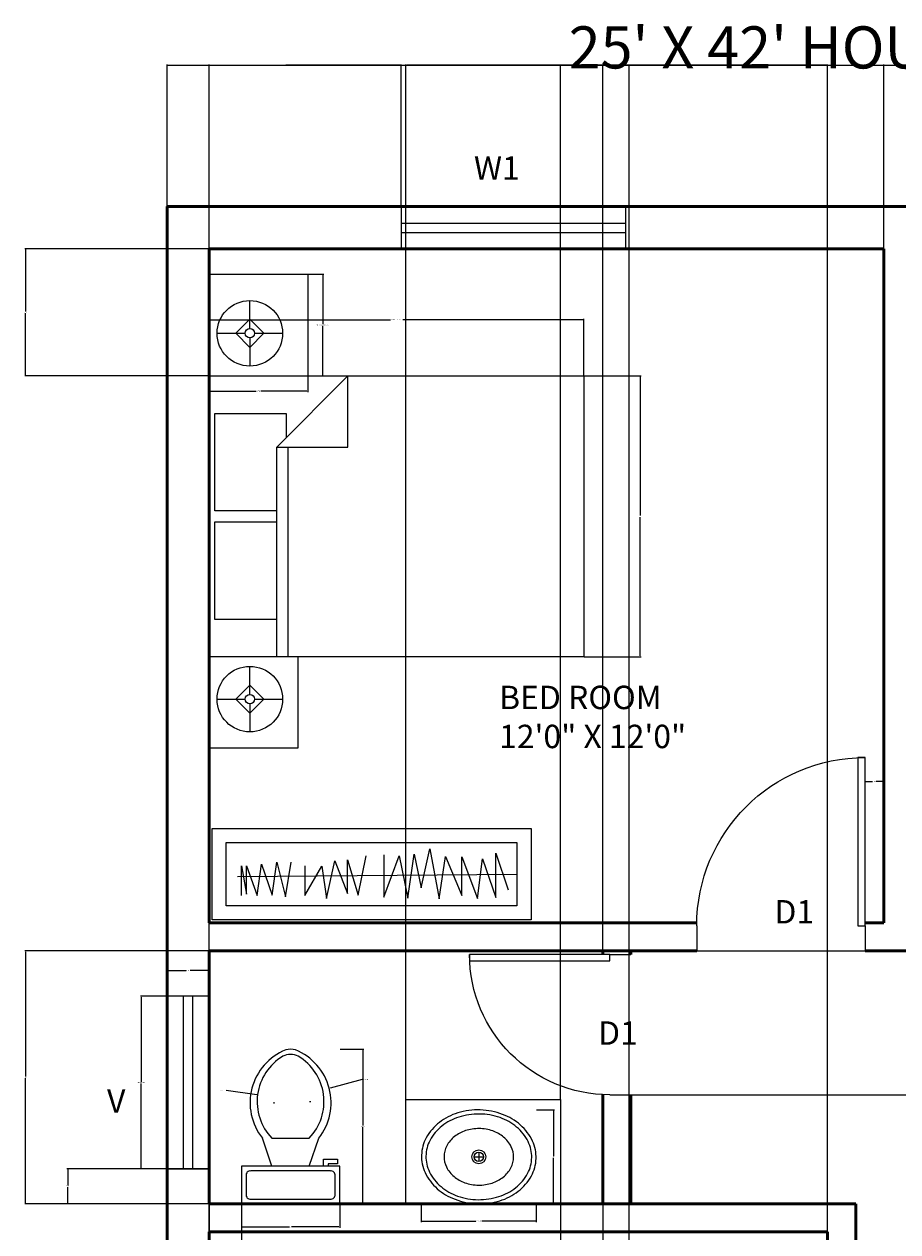
# Model space of a CAD drawing. Units: inches. Extents: x 437 to 811, y 2074 to 2699.
# Tile 3 of 4: x 437 to 624, y 2441 to 2699. Entities that reach past the tile are written whole.
import ezdxf

# ---------------------------------------------------------------- set-up
doc = ezdxf.new("R2010")
doc.units = ezdxf.units.IN
for name, color, linetype, lineweight in [('A-ANNO-DIMS', 2, 'Continuous', 18), ('A-ANNO-TEXT', 7, 'Continuous', 18), ('A-ANNO-TTLB', 7, 'Continuous', 35), ('A-AREA-IDEN', 7, 'Continuous', 25), ('A-DOOR', 4, 'Continuous', 25), ('A-FLOR-CASE', 9, 'Continuous', 25), ('A-FLOR-FIXT', 9, 'Continuous', 18), ('A-FURN', 8, 'Continuous', 18), ('A-GLAZ', 4, 'Continuous', 18), ('A-WALL', 7, 'Continuous', 50)]:
    doc.layers.add(name, color=color, linetype=linetype, lineweight=lineweight)
doc.styles.get("Standard").update_dxf_attribs({"font": 'arial.ttf'})
doc.dimstyles.get("Standard").update_dxf_attribs({"dimtxt": 0.18, "dimasz": 0.18, "dimexe": 0.18, "dimexo": 0.0625, "dimgap": 0.09, "dimtad": 0, "dimtih": 1, "dimtoh": 1, "dimdec": 4, "dimzin": 0, "dimdsep": 46, "dimtxsty": 'Standard', "dimcen": 0.09, "dimadec": 0, "dimazin": 0, "dimtfac": 1, "dimtdec": 4, "dimtofl": 0, "dimtmove": 0, "dimatfit": 3, "dimfxl": 1, "dimtolj": 1, "dimtzin": 0, "dimarcsym": 0})

# ---------------------------------------------------------------- blocks, each defined once
blk = doc.blocks.new('Toilet - top')
for p, q in [((9.5, -6), (9.5, -2)), ((-10, -8.5), (-8, -8.5)), ((-10, -9.5), (-10, -8.5)), ((-7, -9.5), (-10, -9.5)), ((-8, -8.5), (-8, -8)), ((-7, -8), (-7, -9.5)), ((-4, -8), (-6, -14)), ((4, -8), (6, -14)), ((4, -14), (-4, -14))]:
    blk.add_line(p, q)
blk.add_lwpolyline([(10.5, -8), (10.5, 0), (-10.5, 0), (-10.5, -8)], close=True)
for points in [[(-9.5, -2), (-9.5, -6)], [(8.5, -1), (-8.5, -1)], [(-8.5, -7), (8.5, -7)]]:
    blk.add_lwpolyline(points)
for centre, radius, start, end in [((-8.62, -1.88), 0.884, 81.8699, 188.1301), ((8.62, -1.88), 0.884, 351.8699, 98.1301), ((-8.62, -6.12), 0.884, 171.8699, 278.1301), ((8.62, -6.12), 0.884, 261.8699, 8.1301), ((3.52, -21.58), 12.17, 141.4691, 247.9714), ((4.2, -21.82), 11.33, 136.3677, 238.9468), ((-3.52, -21.58), 12.17, 292.0284, 38.5307), ((-4.2, -21.82), 11.33, 301.053, 43.6321), ((0, -27.88), 4, 245.7318, 294.2682), ((0, -29), 4, 254.8605, 285.1395)]:
    blk.add_arc(centre, radius, start, end)
blk = doc.blocks.new('Sink - Oval top')
for p, q in [((-1, 0), (1, 0)), ((0, 1), (0, -1))]:
    blk.add_line(p, q)
for points in [[(-12.23, 0.39, 0.117634), (-11.46, -3.36, 0.104469), (-8.88, -6.8, 0.090016), (-5.08, -9.07, 0.08192), (-0.32, -10.02, 0.08192), (4.49, -9.38, 0.090016), (8.42, -7.36, 0.104469), (11.22, -4.09, 0.117634), (12.23, -0.39, 0.117634), (11.46, 3.36, 0.104469), (8.88, 6.8, 0.090016), (5.08, 9.07, 0.08192), (0.32, 10.02, 0.08192), (-4.49, 9.38, 0.090016), (-8.42, 7.36, 0.104469), (-11.22, 4.09, 0.117634)], [(-11.29, 0.16, 0.118622), (-10.52, -3.25, 0.104678), (-8.07, -6.36, 0.089562), (-4.54, -8.37, 0.081185), (-0.13, -9.15, 0.081185), (4.3, -8.49, 0.089562), (7.89, -6.58, 0.104678), (10.42, -3.55, 0.118622), (11.29, -0.16, 0.118622), (10.52, 3.25, 0.104678), (8.07, 6.36, 0.089562), (4.54, 8.37, 0.081185), (0.13, 9.15, 0.081185), (-4.3, 8.49, 0.089562), (-7.89, 6.58, 0.104678), (-10.42, 3.55, 0.118622)], [(-7.42, 0.08, 0.118283), (-6.91, -2.17, 0.104607), (-5.29, -4.21, 0.089718), (-2.97, -5.53, 0.081436), (-0.07, -6.04, 0.081436), (2.84, -5.59, 0.089718), (5.2, -4.33, 0.104607), (6.86, -2.32, 0.118283), (7.42, -0.08, 0.118283), (6.91, 2.17, 0.104607), (5.29, 4.21, 0.089718), (2.97, 5.53, 0.081436), (0.07, 6.04, 0.081436), (-2.84, 5.59, 0.089718), (-5.2, 4.33, 0.104607), (-6.86, 2.32, 0.118283)]]:
    blk.add_lwpolyline(points, format="xyb", close=True)
for radius in [1.5, 1]:
    blk.add_circle((0, 0), radius)
blk = doc.blocks.new('Bed - Queen')
for p, q in [((0, -80.00003), (0, 0)), ((0, 0), (59.99999, 0)), ((59.99999, 0), (59.99999, -80.00003)), ((7.99999, -1.2), (28.79998, -1.2)), ((7.99999, -14.4), (7.99999, -1.2)), ((28.79998, -1.2), (28.79998, -14.4)), ((31.19999, -1.2), (51.99999, -1.2)), ((31.19999, -14.4), (31.19999, -1.2)), ((51.99999, -1.2), (51.99999, -16.4)), ((0, -14.4), (44.8, -14.4)), ((59.99999, -29.6), (44.8, -14.4)), ((44.8, -14.4), (44.8, -29.6)), ((44.8, -16.8), (0, -16.8)), ((51.99999, -16.4), (46.79936, -16.4)), ((44.8, -29.6), (59.99999, -29.6)), ((59.99999, -80.00003), (0, -80.00003))]:
    blk.add_line(p, q)
blk = doc.blocks.new('Lamp - Table')
for p, q in [((0, 7), (0, 1)), ((0, 3), (-3, 0)), ((3, 0), (0, 3)), ((-1, 0), (-7, 0)), ((-3, 0), (0, -3)), ((0, -3), (3, 0)), ((1, 0), (7, 0)), ((0, -1), (0, -7))]:
    blk.add_line(p, q)
for radius in [7, 1]:
    blk.add_circle((0, 0), radius)
blk = doc.blocks.new('*U10')
for p, q in [((0, 0), (0, -6)), ((40, 0), (40, -6))]:
    blk.add_line(p, q)
blk.add_lwpolyline([(0, 0), (0, 40), (1.75, 40), (1.75, 0)], close=True)
blk.add_arc((0, 0), 40, 0, 90)
blk = doc.blocks.new('WIN-W1-48IN')
for p, q in [((0, 5.5), (48, 5.5)), ((0, 3.5), (48, 3.5))]:
    blk.add_line(p, q)
blk.add_lwpolyline([(0, 0), (48, 0), (48, 9), (0, 9)], close=True)
blk = doc.blocks.new('VENT-V')
for p, q in [((9, 36.83), (0, 36.83)), ((0, 36.83), (0, 0)), ((3.5, 0), (3.5, 36.83)), ((5.5, 0), (5.5, 36.83)), ((9, 0), (9, 36.83)), ((0, 0), (9, 0))]:
    blk.add_line(p, q)
blk = doc.blocks.new('WARDROBE-BEDROOM')
for p, q in [((31.2, 5.25), (32.85, 13.72)), ((36.63, 13.91), (36.63, 4.86)), ((36.63, 4.86), (39.94, 13.72)), ((39.94, 13.72), (41.79, 4.67)), ((41.79, 4.67), (43.13, 14.04)), ((43.13, 14.04), (44.6, 6.84)), ((44.6, 6.84), (46.44, 15.19)), ((46.44, 15.19), (48.48, 4.48)), ((48.48, 4.48), (49.82, 13.53)), ((49.82, 13.53), (53.33, 5.18)), ((53.33, 5.18), (53.33, 13.47)), ((53.33, 13.47), (56.64, 4.54)), ((56.64, 4.54), (57.73, 13.02)), ((57.73, 13.02), (60.53, 4.8)), ((60.53, 4.8), (60.53, 14.29)), ((60.53, 14.29), (63.21, 6.39)), ((6.24, 5.24), (6.24, 11.53)), ((6.24, 11.53), (7.31, 5.48)), ((7.31, 5.48), (7.31, 11.54)), ((7.31, 11.54), (9.63, 5.2)), ((9.63, 5.2), (10.54, 11.9)), ((10.54, 11.9), (12.78, 5.28)), ((12.78, 5.28), (13.81, 12.34)), ((13.81, 12.34), (15.69, 4.96)), ((15.69, 4.96), (16.88, 12.37)), ((19.79, 11.56), (19.79, 5.18)), ((19.79, 5.18), (23.42, 11.48)), ((23.42, 11.48), (24.44, 4.55)), ((24.44, 4.55), (26.22, 12.64)), ((26.22, 12.64), (28.9, 5.63)), ((28.9, 5.63), (28.9, 12.83)), ((28.9, 12.83), (31.2, 5.25)), ((5.43, 9.27), (65.08, 9.77))]:
    blk.add_line(p, q)
for points in [[(0, 19.54), (68.08, 19.54), (68.08, 0), (0, 0)], [(3, 16.54), (65.08, 16.54), (65.08, 3), (3, 3)]]:
    blk.add_lwpolyline(points, close=True)
blk = doc.blocks.new('NIGHTSTAND-SMALL')
for p, q in [((0, 19.48), (0, 0)), ((19, 0), (19, 19.48)), ((0, 0), (19, 0))]:
    blk.add_line(p, q)
blk = doc.blocks.new('NIGHTSTAND-LARGE')
for p, q in [((0, 0), (0, 21.74)), ((0, 21.74), (21.02, 21.74)), ((21.02, 21.74), (21.02, 0))]:
    blk.add_line(p, q)
blk = doc.blocks.new('*D20')
at = {"layer": 'A-ANNO-DIMS', "color": 0, "lineweight": -2, "transparency": 16777216}
for p, q in [((477, 2623.7), (477, 2635.82)), ((477.18, 2635.64), (515.7, 2635.64)), ((556.82, 2635.64), (518.31, 2635.64)), ((557, 2623.7), (557, 2635.82))]:
    blk.add_line(p, q, dxfattribs=at)
at = {"layer": 'A-ANNO-DIMS', "color": 0, "transparency": 16777216}
for points in [[(477.18, 2635.67), (477.18, 2635.61), (477, 2635.64)], [(556.82, 2635.67), (556.82, 2635.61), (557, 2635.64)]]:
    blk.add_solid(points, dxfattribs=at)
at = {"layer": 'Defpoints', "color": 0, "transparency": 16777216}
for p in [(477, 2635.64), (477, 2623.64), (557, 2623.64)]:
    blk.add_point(p, dxfattribs=at)
at = {"layer": 'A-ANNO-DIMS', "color": 0, "transparency": 16777216, "insert": (517, 2635.64), "char_height": 0.18, "attachment_point": 5}
blk.add_mtext('\\A1;QUEEN BED 80 TYP.', dxfattribs=at)
blk = doc.blocks.new('*D21')
at = {"layer": 'A-ANNO-DIMS', "color": 0, "lineweight": -2, "transparency": 16777216}
for p, q in [((557.07, 2623.64), (569.18, 2623.64)), ((569, 2623.46), (569, 2593.82)), ((569, 2563.82), (569, 2593.46)), ((557.07, 2563.64), (569.18, 2563.64))]:
    blk.add_line(p, q, dxfattribs=at)
at = {"layer": 'A-ANNO-DIMS', "color": 0, "transparency": 16777216}
for points in [[(568.97, 2623.46), (569.03, 2623.46), (569, 2623.64)], [(568.97, 2563.82), (569.03, 2563.82), (569, 2563.64)]]:
    blk.add_solid(points, dxfattribs=at)
at = {"layer": 'Defpoints', "color": 0, "transparency": 16777216}
for p in [(557, 2623.64), (569, 2623.64), (557, 2563.64)]:
    blk.add_point(p, dxfattribs=at)
at = {"layer": 'A-ANNO-DIMS', "color": 0, "transparency": 16777216, "insert": (569, 2593.64), "char_height": 0.18, "attachment_point": 5}
blk.add_mtext('\\A1;60 TYP.', dxfattribs=at)
blk = doc.blocks.new('*D24')
at = {"layer": 'A-ANNO-DIMS', "color": 0, "lineweight": -2, "transparency": 16777216}
for p, q in [((498.09, 2645.39), (501.47, 2645.39)), ((501.29, 2645.21), (501.29, 2634.72)), ((501.29, 2623.82), (501.29, 2634.31)), ((498.09, 2623.64), (501.47, 2623.64))]:
    blk.add_line(p, q, dxfattribs=at)
at = {"layer": 'A-ANNO-DIMS', "color": 0, "transparency": 16777216}
for points in [[(501.26, 2645.21), (501.32, 2645.21), (501.29, 2645.39)], [(501.26, 2623.82), (501.32, 2623.82), (501.29, 2623.64)]]:
    blk.add_solid(points, dxfattribs=at)
at = {"layer": 'Defpoints', "color": 0, "transparency": 16777216}
for p in [(498.03, 2645.39), (501.29, 2645.39), (498.03, 2623.64)]:
    blk.add_point(p, dxfattribs=at)
at = {"layer": 'A-ANNO-DIMS', "color": 0, "transparency": 16777216, "insert": (501.29, 2634.51), "char_height": 0.18, "attachment_point": 5}
blk.add_mtext('\\A1;NIGHTSTAND (L) 22 TYP.', dxfattribs=at)
blk = doc.blocks.new('*D25')
at = {"layer": 'A-ANNO-DIMS', "color": 0, "lineweight": -2, "transparency": 16777216}
for p, q in [((477, 2623.58), (477, 2620.2)), ((498.03, 2623.58), (498.03, 2620.2)), ((477.18, 2620.38), (486.99, 2620.38)), ((497.85, 2620.38), (488.05, 2620.38))]:
    blk.add_line(p, q, dxfattribs=at)
at = {"layer": 'A-ANNO-DIMS', "color": 0, "transparency": 16777216}
for points in [[(477.18, 2620.41), (477.18, 2620.35), (477, 2620.38)], [(497.85, 2620.41), (497.85, 2620.35), (498.03, 2620.38)]]:
    blk.add_solid(points, dxfattribs=at)
at = {"layer": 'Defpoints', "color": 0, "transparency": 16777216}
for p in [(477, 2623.64), (498.03, 2623.64), (498.03, 2620.38)]:
    blk.add_point(p, dxfattribs=at)
at = {"layer": 'A-ANNO-DIMS', "color": 0, "transparency": 16777216, "insert": (487.52, 2620.38), "char_height": 0.18, "attachment_point": 5}
blk.add_mtext('\\A1;21 TYP.', dxfattribs=at)
blk = doc.blocks.new('*D28')
at = {"layer": 'A-ANNO-DIMS', "color": 0, "lineweight": -2, "transparency": 16777216}
for p, q in [((467.94, 2491.12), (462.3, 2491.12)), ((462.48, 2490.94), (462.48, 2472.88)), ((462.48, 2454.47), (462.48, 2472.52)), ((467.94, 2454.29), (462.3, 2454.29))]:
    blk.add_line(p, q, dxfattribs=at)
at = {"layer": 'A-ANNO-DIMS', "color": 0, "transparency": 16777216}
for points in [[(462.45, 2490.94), (462.51, 2490.94), (462.48, 2491.12)], [(462.45, 2454.47), (462.51, 2454.47), (462.48, 2454.29)]]:
    blk.add_solid(points, dxfattribs=at)
at = {"layer": 'Defpoints', "color": 0, "transparency": 16777216}
for p in [(462.48, 2491.12), (468, 2491.12), (468, 2454.29)]:
    blk.add_point(p, dxfattribs=at)
at = {"layer": 'A-ANNO-DIMS', "color": 0, "transparency": 16777216, "insert": (462.48, 2472.7), "char_height": 0.18, "attachment_point": 5}
blk.add_mtext('\\A1;VENT 37 TYP.', dxfattribs=at)
blk = doc.blocks.new('*D29')
at = {"layer": 'A-ANNO-DIMS', "color": 0, "lineweight": -2, "transparency": 16777216}
for p, q in [((468, 2491.18), (468, 2496.82)), ((468.18, 2496.64), (472.05, 2496.64)), ((476.82, 2496.64), (472.96, 2496.64)), ((477, 2491.18), (477, 2496.82))]:
    blk.add_line(p, q, dxfattribs=at)
at = {"layer": 'A-ANNO-DIMS', "color": 0, "transparency": 16777216}
for points in [[(468.18, 2496.67), (468.18, 2496.61), (468, 2496.64)], [(476.82, 2496.67), (476.82, 2496.61), (477, 2496.64)]]:
    blk.add_solid(points, dxfattribs=at)
at = {"layer": 'Defpoints', "color": 0, "transparency": 16777216}
for p in [(477, 2496.64), (468, 2491.12), (477, 2491.12)]:
    blk.add_point(p, dxfattribs=at)
at = {"layer": 'A-ANNO-DIMS', "color": 0, "transparency": 16777216, "insert": (472.5, 2496.64), "char_height": 0.18, "attachment_point": 5}
blk.add_mtext('\\A1;9 TYP.', dxfattribs=at)
blk = doc.blocks.new('*D32')
at = {"layer": 'A-ANNO-DIMS', "color": 0, "lineweight": -2, "transparency": 16777216}
for p, q in [((504.93, 2479.85), (510.01, 2479.85)), ((509.83, 2479.67), (509.83, 2463.51)), ((509.83, 2446.98), (509.83, 2463.14)), ((504.93, 2446.8), (510.01, 2446.8))]:
    blk.add_line(p, q, dxfattribs=at)
at = {"layer": 'A-ANNO-DIMS', "color": 0, "transparency": 16777216}
for points in [[(509.8, 2479.67), (509.86, 2479.67), (509.83, 2479.85)], [(509.8, 2446.98), (509.86, 2446.98), (509.83, 2446.8)]]:
    blk.add_solid(points, dxfattribs=at)
at = {"layer": 'Defpoints', "color": 0, "transparency": 16777216}
for p in [(504.87, 2479.85), (504.87, 2446.8), (509.83, 2446.8)]:
    blk.add_point(p, dxfattribs=at)
at = {"layer": 'A-ANNO-DIMS', "color": 0, "transparency": 16777216, "insert": (509.83, 2463.32), "char_height": 0.18, "attachment_point": 5}
blk.add_mtext('\\A1;WC 33', dxfattribs=at)
blk = doc.blocks.new('*D33')
at = {"layer": 'A-ANNO-DIMS', "color": 0, "lineweight": -2, "transparency": 16777216}
for p, q in [((483.87, 2446.74), (483.87, 2441.66)), ((504.87, 2446.74), (504.87, 2441.66)), ((484.05, 2441.84), (494.17, 2441.84)), ((504.69, 2441.84), (494.57, 2441.84))]:
    blk.add_line(p, q, dxfattribs=at)
at = {"layer": 'A-ANNO-DIMS', "color": 0, "transparency": 16777216}
for points in [[(484.05, 2441.87), (484.05, 2441.81), (483.87, 2441.84)], [(504.69, 2441.87), (504.69, 2441.81), (504.87, 2441.84)]]:
    blk.add_solid(points, dxfattribs=at)
at = {"layer": 'Defpoints', "color": 0, "transparency": 16777216}
for p in [(483.87, 2446.8), (504.87, 2446.8), (483.87, 2441.84)]:
    blk.add_point(p, dxfattribs=at)
at = {"layer": 'A-ANNO-DIMS', "color": 0, "transparency": 16777216, "insert": (494.37, 2441.84), "char_height": 0.18, "attachment_point": 5}
blk.add_mtext('\\A1;21', dxfattribs=at)
blk = doc.blocks.new('*D34')
at = {"layer": 'A-ANNO-DIMS', "color": 0, "lineweight": -2, "transparency": 16777216}
for p, q in [((522.28, 2446.69), (522.28, 2442.89)), ((546.83, 2446.69), (546.83, 2442.89)), ((522.46, 2443.07), (533.93, 2443.07)), ((546.65, 2443.07), (535.18, 2443.07))]:
    blk.add_line(p, q, dxfattribs=at)
at = {"layer": 'A-ANNO-DIMS', "color": 0, "transparency": 16777216}
for points in [[(522.46, 2443.1), (522.46, 2443.04), (522.28, 2443.07)], [(546.65, 2443.1), (546.65, 2443.04), (546.83, 2443.07)]]:
    blk.add_solid(points, dxfattribs=at)
at = {"layer": 'Defpoints', "color": 0, "transparency": 16777216}
for p in [(522.28, 2446.75), (546.83, 2446.75), (546.83, 2443.07)]:
    blk.add_point(p, dxfattribs=at)
at = {"layer": 'A-ANNO-DIMS', "color": 0, "transparency": 16777216, "insert": (534.56, 2443.07), "char_height": 0.18, "attachment_point": 5}
blk.add_mtext('\\A1;BASIN 25', dxfattribs=at)
blk = doc.blocks.new('*D35')
at = {"layer": 'A-ANNO-DIMS', "color": 0, "lineweight": -2, "transparency": 16777216}
for p, q in [((546.89, 2466.89), (550.69, 2466.89)), ((550.51, 2466.71), (550.51, 2457)), ((550.51, 2446.93), (550.51, 2456.64)), ((546.89, 2446.75), (550.69, 2446.75))]:
    blk.add_line(p, q, dxfattribs=at)
at = {"layer": 'A-ANNO-DIMS', "color": 0, "transparency": 16777216}
for points in [[(550.48, 2466.71), (550.54, 2466.71), (550.51, 2466.89)], [(550.48, 2446.93), (550.54, 2446.93), (550.51, 2446.75)]]:
    blk.add_solid(points, dxfattribs=at)
at = {"layer": 'Defpoints', "color": 0, "transparency": 16777216}
for p in [(546.83, 2466.89), (550.51, 2466.89), (546.83, 2446.75)]:
    blk.add_point(p, dxfattribs=at)
at = {"layer": 'A-ANNO-DIMS', "color": 0, "transparency": 16777216, "insert": (550.51, 2456.82), "char_height": 0.18, "attachment_point": 5}
blk.add_mtext('\\A1;20', dxfattribs=at)
blk = doc.blocks.new('*D48')
at = {"layer": 'A-ANNO-DIMS', "color": 0, "lineweight": -2, "transparency": 16777216}
for p, q in [((468, 2659.86), (468, 2690.18)), ((468.18, 2690), (492.58, 2690)), ((517.77, 2690), (493.38, 2690)), ((517.95, 2659.86), (517.95, 2690.18))]:
    blk.add_line(p, q, dxfattribs=at)
at = {"layer": 'A-ANNO-DIMS', "color": 0, "transparency": 16777216}
for points in [[(468.18, 2690.03), (468.18, 2689.97), (468, 2690)], [(517.77, 2690.03), (517.77, 2689.97), (517.95, 2690)]]:
    blk.add_solid(points, dxfattribs=at)
at = {"layer": 'Defpoints', "color": 0, "transparency": 16777216}
for p in [(517.95, 2690), (468, 2659.8), (517.95, 2659.8)]:
    blk.add_point(p, dxfattribs=at)
at = {"layer": 'A-ANNO-DIMS', "color": 0, "transparency": 16777216, "insert": (492.98, 2690), "char_height": 0.18, "attachment_point": 5}
blk.add_mtext('\\A1;49.95', dxfattribs=at)
blk = doc.blocks.new('*D50')
at = {"layer": 'A-ANNO-DIMS', "color": 0, "lineweight": -2, "transparency": 16777216}
for p, q in [((621, 2650.86), (621, 2690.18)), ((621.18, 2690), (623.86, 2690)), ((626.82, 2690), (624.15, 2690)), ((627, 2650.86), (627, 2690.18))]:
    blk.add_line(p, q, dxfattribs=at)
at = {"layer": 'A-ANNO-DIMS', "color": 0, "transparency": 16777216}
for points in [[(621.18, 2690.03), (621.18, 2689.97), (621, 2690)], [(626.82, 2690.03), (626.82, 2689.97), (627, 2690)]]:
    blk.add_solid(points, dxfattribs=at)
at = {"layer": 'Defpoints', "color": 0, "transparency": 16777216}
for p in [(627, 2690), (621, 2650.8), (627, 2650.8)]:
    blk.add_point(p, dxfattribs=at)
at = {"layer": 'A-ANNO-DIMS', "color": 0, "transparency": 16777216, "insert": (624, 2690), "char_height": 0.18, "attachment_point": 5}
blk.add_mtext('\\A1;6', dxfattribs=at)
blk = doc.blocks.new('*D54')
at = {"layer": 'A-ANNO-DIMS', "color": 0, "lineweight": -2, "transparency": 16777216}
for p, q in [((476.94, 2454.29), (446.62, 2454.29)), ((446.8, 2454.11), (446.8, 2450.73)), ((446.8, 2446.98), (446.8, 2450.36)), ((476.94, 2446.8), (446.62, 2446.8))]:
    blk.add_line(p, q, dxfattribs=at)
at = {"layer": 'A-ANNO-DIMS', "color": 0, "transparency": 16777216}
for points in [[(446.77, 2454.11), (446.83, 2454.11), (446.8, 2454.29)], [(446.77, 2446.98), (446.83, 2446.98), (446.8, 2446.8)]]:
    blk.add_solid(points, dxfattribs=at)
at = {"layer": 'Defpoints', "color": 0, "transparency": 16777216}
for p in [(446.8, 2454.29), (477, 2454.29), (477, 2446.8)]:
    blk.add_point(p, dxfattribs=at)
at = {"layer": 'A-ANNO-DIMS', "color": 0, "transparency": 16777216, "insert": (446.8, 2450.54), "char_height": 0.18, "attachment_point": 5}
blk.add_mtext('\\A1;7.489', dxfattribs=at)
blk = doc.blocks.new('*D57')
at = {"layer": 'A-ANNO-DIMS', "color": 0, "lineweight": -2, "transparency": 16777216}
for p, q in [((477, 2500.86), (477, 2690.18)), ((477.18, 2690), (518.79, 2690)), ((560.82, 2690), (519.22, 2690)), ((561, 2500.86), (561, 2690.18))]:
    blk.add_line(p, q, dxfattribs=at)
at = {"layer": 'A-ANNO-DIMS', "color": 0, "transparency": 16777216}
for points in [[(477.18, 2690.03), (477.18, 2689.97), (477, 2690)], [(560.82, 2690.03), (560.82, 2689.97), (561, 2690)]]:
    blk.add_solid(points, dxfattribs=at)
at = {"layer": 'Defpoints', "color": 0, "transparency": 16777216}
for p in [(561, 2690), (477, 2500.8), (561, 2500.8)]:
    blk.add_point(p, dxfattribs=at)
at = {"layer": 'A-ANNO-DIMS', "color": 0, "transparency": 16777216, "insert": (519, 2690), "char_height": 0.18, "attachment_point": 5}
blk.add_mtext('\\A1;84', dxfattribs=at)
blk = doc.blocks.new('*D58')
at = {"layer": 'A-ANNO-DIMS', "color": 0, "lineweight": -2, "transparency": 16777216}
for p, q in [((476.94, 2500.8), (437.62, 2500.8)), ((437.8, 2500.62), (437.8, 2473.98)), ((437.8, 2446.98), (437.8, 2473.62)), ((476.94, 2446.8), (437.62, 2446.8))]:
    blk.add_line(p, q, dxfattribs=at)
at = {"layer": 'A-ANNO-DIMS', "color": 0, "transparency": 16777216}
for points in [[(437.77, 2500.62), (437.83, 2500.62), (437.8, 2500.8)], [(437.77, 2446.98), (437.83, 2446.98), (437.8, 2446.8)]]:
    blk.add_solid(points, dxfattribs=at)
at = {"layer": 'Defpoints', "color": 0, "transparency": 16777216}
for p in [(437.8, 2500.8), (477, 2500.8), (477, 2446.8)]:
    blk.add_point(p, dxfattribs=at)
at = {"layer": 'A-ANNO-DIMS', "color": 0, "transparency": 16777216, "insert": (437.8, 2473.8), "char_height": 0.18, "attachment_point": 5}
blk.add_mtext('\\A1;54', dxfattribs=at)
blk = doc.blocks.new('*D59')
at = {"layer": 'A-ANNO-DIMS', "color": 0, "lineweight": -2, "transparency": 16777216}
for p, q in [((567.07, 2500.8), (810.38, 2500.8)), ((810.2, 2500.62), (810.2, 2485.62)), ((810.2, 2470.27), (810.2, 2485.26)), ((567.07, 2470.09), (810.38, 2470.09))]:
    blk.add_line(p, q, dxfattribs=at)
at = {"layer": 'A-ANNO-DIMS', "color": 0, "transparency": 16777216}
for points in [[(810.17, 2500.62), (810.23, 2500.62), (810.2, 2500.8)], [(810.17, 2470.27), (810.23, 2470.27), (810.2, 2470.09)]]:
    blk.add_solid(points, dxfattribs=at)
at = {"layer": 'Defpoints', "color": 0, "transparency": 16777216}
for p in [(567, 2500.8), (810.2, 2500.8), (567, 2470.09)]:
    blk.add_point(p, dxfattribs=at)
at = {"layer": 'A-ANNO-DIMS', "color": 0, "transparency": 16777216, "insert": (810.2, 2485.44), "char_height": 0.18, "attachment_point": 5}
blk.add_mtext('\\A1;30.714', dxfattribs=at)
blk = doc.blocks.new('*D66')
at = {"layer": 'A-ANNO-DIMS', "color": 0, "lineweight": -2, "transparency": 16777216}
for p, q in [((477, 2302.86), (477, 2690.18)), ((477.18, 2690), (542.73, 2690)), ((608.82, 2690), (543.28, 2690)), ((609, 2302.86), (609, 2690.18))]:
    blk.add_line(p, q, dxfattribs=at)
at = {"layer": 'A-ANNO-DIMS', "color": 0, "transparency": 16777216}
for points in [[(477.18, 2690.03), (477.18, 2689.97), (477, 2690)], [(608.82, 2690.03), (608.82, 2689.97), (609, 2690)]]:
    blk.add_solid(points, dxfattribs=at)
at = {"layer": 'Defpoints', "color": 0, "transparency": 16777216}
for p in [(609, 2690), (477, 2302.8), (609, 2302.8)]:
    blk.add_point(p, dxfattribs=at)
at = {"layer": 'A-ANNO-DIMS', "color": 0, "transparency": 16777216, "insert": (543, 2690), "char_height": 0.18, "attachment_point": 5}
blk.add_mtext('\\A1;132', dxfattribs=at)
blk = doc.blocks.new('*D69')
at = {"layer": 'A-ANNO-DIMS', "color": 0, "lineweight": -2, "transparency": 16777216}
for p, q in [((566.64, 2244.86), (566.64, 2690.18)), ((566.82, 2690), (587.42, 2690)), ((608.82, 2690), (588.22, 2690)), ((609, 2247.25), (609, 2690.18))]:
    blk.add_line(p, q, dxfattribs=at)
at = {"layer": 'A-ANNO-DIMS', "color": 0, "transparency": 16777216}
for points in [[(566.82, 2690.03), (566.82, 2689.97), (566.64, 2690)], [(608.82, 2690.03), (608.82, 2689.97), (609, 2690)]]:
    blk.add_solid(points, dxfattribs=at)
at = {"layer": 'Defpoints', "color": 0, "transparency": 16777216}
for p in [(609, 2690), (609, 2247.18), (566.64, 2244.8)]:
    blk.add_point(p, dxfattribs=at)
at = {"layer": 'A-ANNO-DIMS', "color": 0, "transparency": 16777216, "insert": (587.82, 2690), "char_height": 0.18, "attachment_point": 5}
blk.add_mtext('\\A1;42.37', dxfattribs=at)
blk = doc.blocks.new('*D71')
at = {"layer": 'A-ANNO-DIMS', "color": 0, "lineweight": -2, "transparency": 16777216}
for p, q in [((477, 2446.74), (477, 2074.42)), ((483.87, 2446.74), (483.87, 2074.42)), ((477.18, 2074.6), (480.04, 2074.6)), ((483.69, 2074.6), (480.83, 2074.6))]:
    blk.add_line(p, q, dxfattribs=at)
at = {"layer": 'A-ANNO-DIMS', "color": 0, "transparency": 16777216}
for points in [[(477.18, 2074.63), (477.18, 2074.57), (477, 2074.6)], [(483.69, 2074.63), (483.69, 2074.57), (483.87, 2074.6)]]:
    blk.add_solid(points, dxfattribs=at)
at = {"layer": 'Defpoints', "color": 0, "transparency": 16777216}
for p in [(477, 2446.8), (483.87, 2446.8), (483.87, 2074.6)]:
    blk.add_point(p, dxfattribs=at)
at = {"layer": 'A-ANNO-DIMS', "color": 0, "transparency": 16777216, "insert": (480.44, 2074.6), "char_height": 0.18, "attachment_point": 5}
blk.add_mtext('\\A1;6.864', dxfattribs=at)
blk = doc.blocks.new('*D72')
at = {"layer": 'A-ANNO-DIMS', "color": 0, "lineweight": -2, "transparency": 16777216}
for p, q in [((519, 2469.12), (519, 2690.18)), ((519.18, 2690), (535.02, 2690)), ((551.78, 2690), (535.95, 2690)), ((551.96, 2469.12), (551.96, 2690.18))]:
    blk.add_line(p, q, dxfattribs=at)
at = {"layer": 'A-ANNO-DIMS', "color": 0, "transparency": 16777216}
for points in [[(519.18, 2690.03), (519.18, 2689.97), (519, 2690)], [(551.78, 2690.03), (551.78, 2689.97), (551.96, 2690)]]:
    blk.add_solid(points, dxfattribs=at)
at = {"layer": 'Defpoints', "color": 0, "transparency": 16777216}
for p in [(551.96, 2690), (519, 2469.06), (551.96, 2469.06)]:
    blk.add_point(p, dxfattribs=at)
at = {"layer": 'A-ANNO-DIMS', "color": 0, "transparency": 16777216, "insert": (535.48, 2690), "char_height": 0.18, "attachment_point": 5}
blk.add_mtext('\\A1;32.955', dxfattribs=at)
blk = doc.blocks.new('*D73')
at = {"layer": 'A-ANNO-DIMS', "color": 0, "lineweight": -2, "transparency": 16777216}
for p, q in [((551.96, 2446.74), (551.96, 2074.42)), ((561, 2446.74), (561, 2074.42)), ((552.14, 2074.6), (556.09, 2074.6)), ((560.82, 2074.6), (556.88, 2074.6))]:
    blk.add_line(p, q, dxfattribs=at)
at = {"layer": 'A-ANNO-DIMS', "color": 0, "transparency": 16777216}
for points in [[(552.14, 2074.63), (552.14, 2074.57), (551.96, 2074.6)], [(560.82, 2074.63), (560.82, 2074.57), (561, 2074.6)]]:
    blk.add_solid(points, dxfattribs=at)
at = {"layer": 'Defpoints', "color": 0, "transparency": 16777216}
for p in [(551.96, 2446.8), (561, 2446.8), (561, 2074.6)]:
    blk.add_point(p, dxfattribs=at)
at = {"layer": 'A-ANNO-DIMS', "color": 0, "transparency": 16777216, "insert": (556.48, 2074.6), "char_height": 0.18, "attachment_point": 5}
blk.add_mtext('\\A1;9.045', dxfattribs=at)
blk = doc.blocks.new('*D75')
at = {"layer": 'A-ANNO-DIMS', "color": 0, "lineweight": -2, "transparency": 16777216}
for p, q in [((617, 2506.86), (617, 2537.18)), ((617.18, 2537), (618.62, 2537)), ((620.82, 2537), (619.38, 2537)), ((621, 2506.86), (621, 2537.18))]:
    blk.add_line(p, q, dxfattribs=at)
at = {"layer": 'A-ANNO-DIMS', "color": 0, "transparency": 16777216}
for points in [[(617.18, 2537.03), (617.18, 2536.97), (617, 2537)], [(620.82, 2537.03), (620.82, 2536.97), (621, 2537)]]:
    blk.add_solid(points, dxfattribs=at)
at = {"layer": 'Defpoints', "color": 0, "transparency": 16777216}
for p in [(621, 2537), (617, 2506.8), (621, 2506.8)]:
    blk.add_point(p, dxfattribs=at)
at = {"layer": 'A-ANNO-DIMS', "color": 0, "transparency": 16777216, "insert": (619, 2537), "char_height": 0.18, "attachment_point": 5}
blk.add_mtext('\\A1;4.001', dxfattribs=at)
blk = doc.blocks.new('*D79')
at = {"layer": 'A-ANNO-DIMS', "color": 0, "lineweight": -2, "transparency": 16777216}
for p, q in [((476.94, 2650.8), (437.62, 2650.8)), ((437.8, 2650.62), (437.8, 2637.4)), ((437.8, 2623.82), (437.8, 2637.04)), ((476.94, 2623.64), (437.62, 2623.64))]:
    blk.add_line(p, q, dxfattribs=at)
at = {"layer": 'A-ANNO-DIMS', "color": 0, "transparency": 16777216}
for points in [[(437.77, 2650.62), (437.83, 2650.62), (437.8, 2650.8)], [(437.77, 2623.82), (437.83, 2623.82), (437.8, 2623.64)]]:
    blk.add_solid(points, dxfattribs=at)
at = {"layer": 'Defpoints', "color": 0, "transparency": 16777216}
for p in [(477, 2650.8), (437.8, 2623.64), (477, 2623.64)]:
    blk.add_point(p, dxfattribs=at)
at = {"layer": 'A-ANNO-DIMS', "color": 0, "transparency": 16777216, "insert": (437.8, 2637.22), "char_height": 0.18, "attachment_point": 5}
blk.add_mtext('\\A1;27.16', dxfattribs=at)
blk = doc.blocks.new('*D86')
at = {"layer": 'A-ANNO-DIMS', "color": 0, "lineweight": -2, "transparency": 16777216}
for p, q in [((468, 2659.86), (468, 2690.18)), ((468.18, 2690), (623.72, 2690)), ((779.82, 2690), (624.29, 2690)), ((780, 2659.86), (780, 2690.18))]:
    blk.add_line(p, q, dxfattribs=at)
at = {"layer": 'A-ANNO-DIMS', "color": 0, "transparency": 16777216}
for points in [[(468.18, 2690.03), (468.18, 2689.97), (468, 2690)], [(779.82, 2690.03), (779.82, 2689.97), (780, 2690)]]:
    blk.add_solid(points, dxfattribs=at)
at = {"layer": 'Defpoints', "color": 0, "transparency": 16777216}
for p in [(780, 2690), (468, 2659.8), (780, 2659.8)]:
    blk.add_point(p, dxfattribs=at)
at = {"layer": 'A-ANNO-DIMS', "color": 0, "transparency": 16777216, "insert": (624, 2690), "char_height": 0.18, "attachment_point": 5}
blk.add_mtext('\\A1;312', dxfattribs=at)
blk = doc.blocks.new('*D92')
at = {"layer": 'A-ANNO-DIMS', "color": 0, "lineweight": -2, "transparency": 16777216}
for p, q in [((509.68, 2473.33), (502.79, 2471.52)), ((490.76, 2468.38), (490.94, 2468.38)), ((490.85, 2468.29), (490.85, 2468.47))]:
    blk.add_line(p, q, dxfattribs=at)
at = {"layer": 'A-ANNO-DIMS', "color": 0, "transparency": 16777216}
blk.add_solid([(502.79, 2471.55), (502.8, 2471.49), (502.62, 2471.47)], dxfattribs=at)
at = {"layer": 'Defpoints', "color": 0, "transparency": 16777216}
for p in [(502.62, 2471.47), (490.85, 2468.38)]:
    blk.add_point(p, dxfattribs=at)
at = {"layer": 'A-ANNO-DIMS', "color": 0, "transparency": 16777216, "insert": (510.36, 2473.33), "char_height": 0.18, "attachment_point": 5}
blk.add_mtext('\\A1;2X R12.17', dxfattribs=at)
blk = doc.blocks.new('*D93')
at = {"layer": 'A-ANNO-DIMS', "color": 0, "lineweight": -2, "transparency": 16777216}
for p, q in [((480.6, 2471.03), (487.16, 2470.15)), ((498.48, 2468.62), (498.66, 2468.62)), ((498.57, 2468.53), (498.57, 2468.71))]:
    blk.add_line(p, q, dxfattribs=at)
at = {"layer": 'A-ANNO-DIMS', "color": 0, "transparency": 16777216}
blk.add_solid([(487.17, 2470.18), (487.16, 2470.12), (487.34, 2470.13)], dxfattribs=at)
at = {"layer": 'Defpoints', "color": 0, "transparency": 16777216}
for p in [(487.34, 2470.13), (498.57, 2468.62)]:
    blk.add_point(p, dxfattribs=at)
at = {"layer": 'A-ANNO-DIMS', "color": 0, "transparency": 16777216, "insert": (479.93, 2471.03), "char_height": 0.18, "attachment_point": 5}
blk.add_mtext('\\A1;2X R11.33', dxfattribs=at)

msp = doc.modelspace()

# ---------------------------------------------------------------- linework, layer by layer
at = {"layer": 'A-FLOR-CASE'}
for p, q in [((519.0049, 2446.7995), (519.0049, 2469.0598)), ((519.0049, 2469.0598), (551.9595, 2469.0598)), ((551.9595, 2469.0598), (551.9595, 2446.7995))]:
    msp.add_line(p, q, dxfattribs=at)
at = {"layer": 'A-WALL'}
for p, q in [((468.0049, 2659.7995), (468.0049, 2128.7995)), ((780.0049, 2659.7995), (468.0049, 2659.7995)), ((477.0049, 2650.7995), (477.0049, 2506.7995)), ((621.0049, 2650.7995), (477.0049, 2650.7995)), ((621.0049, 2506.7995), (621.0049, 2650.7995)), ((477.0049, 2506.7995), (581.0847, 2506.7995)), ((617.0035, 2506.7995), (621.0049, 2506.7995)), ((477.0049, 2500.7995), (581.0795, 2500.7995)), ((477.0049, 2500.7995), (477.0049, 2446.7995)), ((561.0049, 2500.0288), (561.0049, 2500.7995)), ((567.0049, 2500.0288), (567.0049, 2500.7995)), ((617.0035, 2500.7995), (631.6694, 2500.7995)), ((561.0049, 2446.7995), (561.0049, 2470.1239)), ((567.0049, 2446.7995), (567.0049, 2470.0858)), ((477.0049, 2446.7995), (561.0049, 2446.7995)), ((615.0049, 2446.7995), (561.0049, 2446.7995)), ((615.0049, 2350.1394), (615.0049, 2446.7995)), ((477.0049, 2440.7995), (561.0049, 2440.7995)), ((477.0049, 2440.7995), (477.0049, 2308.7995)), ((609.0049, 2440.7995), (561.0049, 2440.7995)), ((609.0049, 2350.1342), (609.0049, 2440.7995))]:
    msp.add_line(p, q, dxfattribs=at)

# ---------------------------------------------------------------- block references
at = {"layer": 'A-DOOR', "xscale": -0.8981017077080947, "yscale": 0.8981017077080947, "zscale": 0.8981017077080947}
msp.add_blockref('*U10', (617.0035, 2506.1881), dxfattribs=at)
at = {"layer": 'A-DOOR', "xscale": -0.7485748686315713, "yscale": 0.7485748686315713, "zscale": 0.7485748686315713, "rotation": 90}
msp.add_blockref('*U10', (562.5134, 2500.0288), dxfattribs=at)
at = {"layer": 'A-FLOR-FIXT', "rotation": 180}
msp.add_blockref('Toilet - top', (494.3691, 2446.7995), dxfattribs=at)
at = {"layer": 'A-FLOR-FIXT'}
msp.add_blockref('Sink - Oval top', (534.556, 2456.823), dxfattribs=at)
at = {"layer": 'A-FURN'}
for name, p in [('NIGHTSTAND-LARGE', (477.005, 2623.641)), ('NIGHTSTAND-SMALL', (477.005, 2544.159)), ('WARDROBE-BEDROOM', (477.625, 2507.434))]:
    msp.add_blockref(name, p, dxfattribs=at)
at = {"layer": 'A-FURN', "rotation": 90}
for name, p in [('Lamp - Table', (485.6767, 2632.7401)), ('Bed - Queen', (477.0049, 2563.6406)), ('Lamp - Table', (485.6767, 2554.5958))]:
    msp.add_blockref(name, p, dxfattribs=at)
at = {"layer": 'A-GLAZ'}
for name, p in [('WIN-W1-48IN', (517.951, 2650.799)), ('VENT-V', (468.005, 2454.288))]:
    msp.add_blockref(name, p, dxfattribs=at)

# ---------------------------------------------------------------- texts
at = {"layer": 'A-ANNO-TEXT', "char_height": 5, "width": 52.048983, "attachment_point": 1}
for s, insert in [('W1', (533.5189, 2670.5384)), ('D1', (597.6642, 2511.6712)), ('D1', (560.0095, 2485.7656)), ('V', (455.1862, 2471.2405))]:
    msp.add_mtext(s, dxfattribs=dict(at, insert=insert))
at = {"layer": 'A-ANNO-TTLB', "insert": (553.7348, 2698.3139), "char_height": 9, "width": 177.859247, "attachment_point": 1}
msp.add_mtext("25' X 42' HOUSE PLAN", dxfattribs=at)
at = {"layer": 'A-AREA-IDEN', "insert": (538.8798, 2557.4575), "char_height": 5, "width": 52.048983, "attachment_point": 1}
msp.add_mtext('BED ROOM\\P12\'0" X 12\'0"', dxfattribs=at)

# ---------------------------------------------------------------- dimensions: what is measured, and where the dimension line sits
at = {"layer": 'A-ANNO-DIMS'}
for base, p1, p2, override, picture, middle in [((517.9507, 2689.9995), (468.0049, 2659.7995), (517.9507, 2659.7995), {"dimdec": 2, "dimlfac": 1, "dimrnd": 0, "dimzin": 0, "dimdsep": 46, "dimlunit": 2}, '*D48', (492.9778, 2689.9995)), ((780.0049, 2689.9995), (468.0049, 2659.7995), (780.0049, 2659.7995), {"dimdec": 0, "dimlfac": 1, "dimrnd": 0, "dimzin": 0, "dimdsep": 46, "dimlunit": 2}, '*D86', (624.0049, 2689.9995)), ((561.0049, 2689.9995), (477.0049, 2500.7995), (561.0049, 2500.7995), {"dimdec": 0, "dimlfac": 1, "dimrnd": 0, "dimzin": 0, "dimdsep": 46, "dimlunit": 2}, '*D57', (519.0049, 2689.9995)), ((609.0049, 2689.9995), (477.0049, 2302.7995), (609.0049, 2302.7995), {"dimdec": 0, "dimlfac": 1, "dimrnd": 0, "dimzin": 0, "dimdsep": 46, "dimlunit": 2}, '*D66', (543.0049, 2689.9995)), ((551.9595, 2689.9995), (519.0049, 2469.0598), (551.9595, 2469.0598), {"dimdec": 3, "dimlfac": 1, "dimrnd": 0, "dimzin": 0, "dimdsep": 46, "dimlunit": 2}, '*D72', (535.4822, 2689.9995)), ((609.0049, 2689.9995), (566.639, 2244.7994), (609.0049, 2247.1838), {"dimdec": 2, "dimlfac": 1, "dimrnd": 0, "dimzin": 0, "dimdsep": 46, "dimlunit": 2}, '*D69', (587.8219, 2689.9995)), ((627.0049, 2689.9995), (621.0049, 2650.7995), (627.0049, 2650.7995), {"dimdec": 0, "dimlfac": 1, "dimrnd": 0, "dimzin": 0, "dimdsep": 46, "dimlunit": 2}, '*D50', (624.0049, 2689.9995)), ((621.0049, 2536.9995), (617.0035, 2506.7995), (621.0049, 2506.7995), {"dimdec": 3, "dimlfac": 1, "dimrnd": 0, "dimzin": 0, "dimdsep": 46, "dimlunit": 2}, '*D75', (619.0042, 2536.9995)), ((483.8691, 2074.5995), (477.0049, 2446.7995), (483.8691, 2446.7995), {"dimdec": 3, "dimlfac": 1, "dimrnd": 0, "dimzin": 0, "dimdsep": 46, "dimlunit": 2}, '*D71', (480.437, 2074.5995)), ((561.0049, 2074.5995), (551.9595, 2446.7995), (561.0049, 2446.7995), {"dimdec": 3, "dimlfac": 1, "dimrnd": 0, "dimzin": 0, "dimdsep": 46, "dimlunit": 2}, '*D73', (556.4822, 2074.5995))]:
    dim = msp.add_linear_dim(base=base, p1=p1, p2=p2, dimstyle='Standard', override=override, dxfattribs=at)
    dim.commit()
    dim.dimension.update_dxf_attribs({"geometry": picture, "text_midpoint": middle})
for base, p1, p2, angle, override, picture, middle in [((437.8049, 2623.6406), (477.0049, 2650.7995), (477.0049, 2623.6406), 90, {"dimdec": 2, "dimlfac": 1, "dimrnd": 0, "dimzin": 0, "dimdsep": 46, "dimlunit": 2}, '*D79', (437.8049, 2637.22)), ((437.8049, 2500.7995), (477.0049, 2446.7995), (477.0049, 2500.7995), 90, {"dimdec": 0, "dimlfac": 1, "dimrnd": 0, "dimzin": 0, "dimdsep": 46, "dimlunit": 2}, '*D58', (437.8049, 2473.7995)), ((810.2049, 2500.7995), (567.0049, 2470.0858), (567.0049, 2500.7995), 90, {"dimdec": 3, "dimlfac": 1, "dimrnd": 0, "dimzin": 0, "dimdsep": 46, "dimlunit": 2}, '*D59', (810.2049, 2485.4426)), ((550.5141, 2466.8913), (546.8315, 2446.7547), (546.8315, 2466.8913), 90, {"dimdec": 0, "dimlfac": 1, "dimrnd": 0, "dimzin": 0, "dimdsep": 46, "dimlunit": 2}, '*D35', (550.5141, 2456.823)), ((446.8049, 2454.2882), (477.0049, 2446.7995), (477.0049, 2454.2882), 90, {"dimdec": 3, "dimlfac": 1, "dimrnd": 0, "dimzin": 0, "dimdsep": 46, "dimlunit": 2}, '*D54', (446.8049, 2450.5438)), ((483.8691, 2441.8425), (504.8691, 2446.7995), (483.8691, 2446.7995), 180, {"dimdec": 0, "dimlfac": 1, "dimrnd": 0, "dimzin": 0, "dimdsep": 46, "dimlunit": 2}, '*D33', (494.3691, 2441.8425))]:
    dim = msp.add_linear_dim(base=base, p1=p1, p2=p2, angle=angle, dimstyle='Standard', override=override, dxfattribs=at)
    dim.commit()
    dim.dimension.update_dxf_attribs({"geometry": picture, "text_midpoint": middle})
for base, p1, p2, angle, text, picture, middle in [((501.289, 2645.3858), (498.0272, 2623.6406), (498.0272, 2645.3858), 90, 'NIGHTSTAND (L) <> TYP.', '*D24', (501.289, 2634.5132)), ((477.0049, 2635.6406), (557.0049, 2623.6406), (477.0049, 2623.6406), 180, 'QUEEN BED <> TYP.', '*D20', (517.0049, 2635.6406)), ((569.0049, 2623.6406), (557.0049, 2563.6406), (557.0049, 2623.6406), 90, '<> TYP.', '*D21', (569.0049, 2593.6406)), ((462.4806, 2491.1168), (468.0049, 2454.2882), (468.0049, 2491.1168), 90, 'VENT <> TYP.', '*D28', (462.4806, 2472.7025)), ((509.826, 2446.7995), (504.8691, 2479.8457), (504.8691, 2446.7995), 270, 'WC <>', '*D32', (509.826, 2463.3226))]:
    dim = msp.add_linear_dim(base=base, p1=p1, p2=p2, angle=angle, text=text, dimstyle='Standard', override={"dimdec": 0, "dimlfac": 1, "dimrnd": 0, "dimzin": 0, "dimdsep": 46, "dimlunit": 2}, dxfattribs=at)
    dim.commit()
    dim.dimension.update_dxf_attribs({"geometry": picture, "text_midpoint": middle})
for base, p1, p2, text, picture, middle in [((498.0272, 2620.3788), (477.0049, 2623.6406), (498.0272, 2623.6406), '<> TYP.', '*D25', (487.516, 2620.3788)), ((477.0049, 2496.6411), (468.0049, 2491.1168), (477.0049, 2491.1168), '<> TYP.', '*D29', (472.5049, 2496.6411)), ((546.8315, 2443.0721), (522.2806, 2446.7547), (546.8315, 2446.7547), 'BASIN <>', '*D34', (534.556, 2443.0721))]:
    dim = msp.add_linear_dim(base=base, p1=p1, p2=p2, text=text, dimstyle='Standard', override={"dimdec": 0, "dimlfac": 1, "dimrnd": 0, "dimzin": 0, "dimdsep": 46, "dimlunit": 2}, dxfattribs=at)
    dim.commit()
    dim.dimension.update_dxf_attribs({"geometry": picture, "text_midpoint": middle})
for center, mpoint, picture, middle in [((490.8495, 2468.3799), (502.6191, 2471.472), '*D92', (509.6809, 2473.3273)), ((498.569, 2468.6168), (487.3407, 2470.126), '*D93', (480.6038, 2471.0316))]:
    dim = msp.add_radius_dim(center=center, mpoint=mpoint, text='2X <>', dimstyle='Standard', override={"dimdec": 2, "dimlfac": 1, "dimrnd": 0, "dimzin": 0, "dimdsep": 46, "dimlunit": 2}, dxfattribs=at)
    dim.commit()
    dim.dimension.update_dxf_attribs({"geometry": picture, "text_midpoint": middle, "dimtype": 164})

doc.saveas('drawing.dxf')
